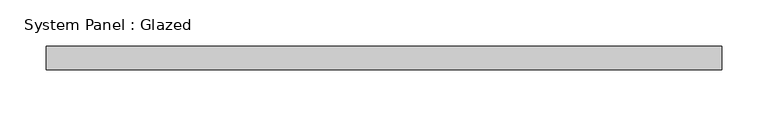
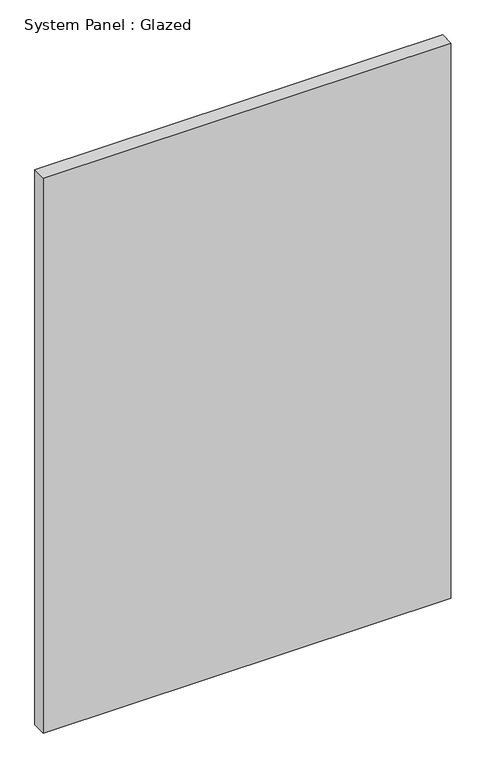
"""IFC4 building model written with IfcOpenShell, lengths in millimetres: plate geometry, System Panel : Glazed."""

from ifc_helpers import new_model, si_unit, origin, origin_with_axes, place, context, project, spatial, polyline, outline, extrude, source, transform, mapped, element, save


def system_panel_glazed_22ff1419(model_context):
    return source(origin(), model_context, "Body", "SweptSolid", [
        extrude(outline(polyline([(366.1833333, 19.05), (-366.1833333, 19.05), (-366.1833333, 44.45), (366.1833333, 44.45), (366.1833333, 19.05)])), origin_with_axes(), (0.0, 0.0, 1.0), 1054.1),
    ])


if __name__ == "__main__":
    model = new_model("IFC4")
    model_context = context("Model", 3, world=origin())
    ifc_project = project(units=[si_unit("LENGTHUNIT", "METRE", prefix="MILLI")], contexts=[model_context])
    site = spatial("IfcSite", under=ifc_project)
    building = spatial("IfcBuilding", under=site)
    placement = place(None, origin())
    system_panel_glazed_shape = system_panel_glazed_22ff1419(model_context)
    element("IfcPlate", 1, ObjectType="System Panel : Glazed", at=placement, inside=building, context=model_context, shape_type="MappedRepresentation", body=[
        mapped(system_panel_glazed_shape, transform((0.0, 0.0, 0.0), x_axis=(1.0, 0.0, 0.0), y_axis=(0.0, 1.0, 0.0), z_axis=(0.0, 0.0, 1.0))),
    ])
    save(model, "model.ifc")

# Revit data of these elements
# Type "System Panel : Glazed"
#   Construction Type Id = "GSP4R"
#   Analytic Construction = "1/8 in Pilkington single glazing"
#   Visual Light Transmittance = 0.9
#   Solar Heat Gain Coefficient = 0.86
#   Heat Transfer Coefficient (U) = 1.18115 BTU/(h·ft²·°F)
# Element 1 (IfcPlate, "System Panel : Glazed")
#   Materials on its faces: "Glass"
# Materials
#   "Glass": class "Glass", colour RGB 0 128 192, transparency 0.75, Description = "Soda Lime Glass", Cost = 0
